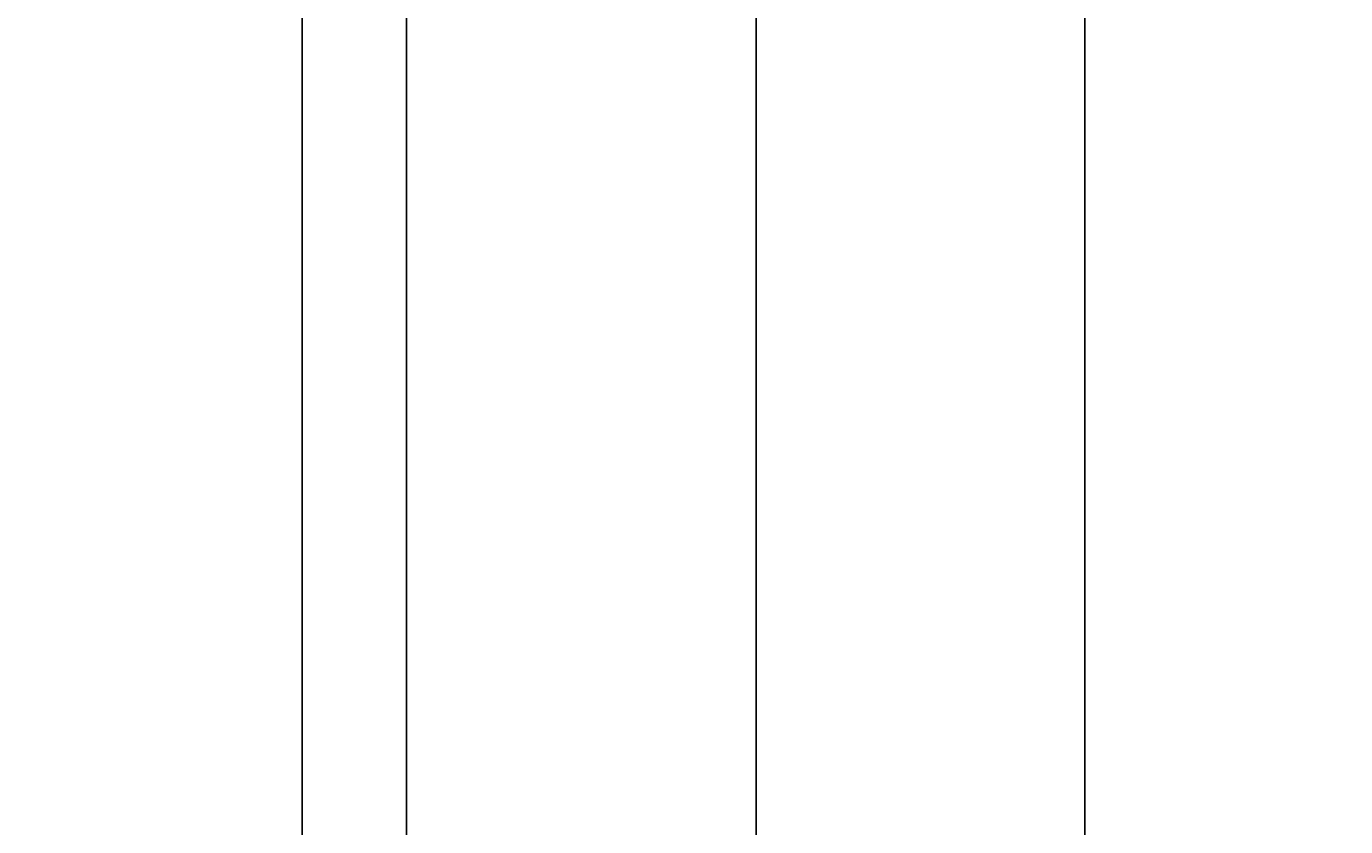
# Model space of a CAD drawing. Units: inches. Extents: x 2231 to 2461, y 2045 to 2455.
# Tile 54 of 95: x 2320 to 2371, y 2271 to 2302. Entities that reach past the tile are written whole.
import ezdxf

# ---------------------------------------------------------------- set-up
doc = ezdxf.new("R2010")
doc.units = ezdxf.units.IN
doc.layers.add('A-ANNO-DIMS', color=2, linetype='Continuous', lineweight=18)
doc.styles.get("Standard").update_dxf_attribs({"font": 'arial.ttf'})
doc.dimstyles.get("Standard").update_dxf_attribs({"dimtxt": 0.18, "dimasz": 0.18, "dimexe": 0.18, "dimexo": 0.0625, "dimgap": 0.09, "dimtad": 0, "dimtih": 1, "dimtoh": 1, "dimdec": 4, "dimzin": 0, "dimdsep": 46, "dimtxsty": 'Standard', "dimcen": 0.09, "dimadec": 0, "dimazin": 0, "dimtfac": 1, "dimtdec": 4, "dimtofl": 0, "dimtmove": 0, "dimatfit": 3, "dimfxl": 1, "dimtolj": 1, "dimtzin": 0, "dimarcsym": 0})

# ---------------------------------------------------------------- blocks, each defined once
blk = doc.blocks.new('*D50')
at = {"layer": 'A-ANNO-DIMS', "color": 0, "lineweight": -2, "transparency": 16777216}
for p, q in [((2304.794, 2182.895), (2304.794, 2454.645)), ((2334.794, 2182.895), (2334.794, 2454.645)), ((2304.974, 2454.465), (2319.575, 2454.465)), ((2334.614, 2454.465), (2320.012, 2454.465))]:
    blk.add_line(p, q, dxfattribs=at)
at = {"layer": 'A-ANNO-DIMS', "color": 0, "transparency": 16777216}
for points in [[(2304.974, 2454.495), (2304.974, 2454.435), (2304.794, 2454.465)], [(2334.614, 2454.495), (2334.614, 2454.435), (2334.794, 2454.465)]]:
    blk.add_solid(points, dxfattribs=at)
at = {"layer": 'Defpoints', "color": 0, "transparency": 16777216}
for p in [(2334.794, 2454.465), (2304.794, 2182.833), (2334.794, 2182.833)]:
    blk.add_point(p, dxfattribs=at)
at = {"layer": 'A-ANNO-DIMS', "color": 0, "transparency": 16777216, "insert": (2319.794, 2454.465), "char_height": 0.18, "attachment_point": 5}
blk.add_mtext('\\A1;30', dxfattribs=at)
blk = doc.blocks.new('*D51')
at = {"layer": 'A-ANNO-DIMS', "color": 0, "lineweight": -2, "transparency": 16777216}
for p, q in [((2258.794, 2306.77), (2258.794, 2044.803)), ((2330.794, 2306.77), (2330.794, 2044.803)), ((2258.974, 2044.983), (2294.576, 2044.983)), ((2330.614, 2044.983), (2295.011, 2044.983))]:
    blk.add_line(p, q, dxfattribs=at)
at = {"layer": 'A-ANNO-DIMS', "color": 0, "transparency": 16777216}
for points in [[(2258.974, 2045.013), (2258.974, 2044.953), (2258.794, 2044.983)], [(2330.614, 2045.013), (2330.614, 2044.953), (2330.794, 2044.983)]]:
    blk.add_solid(points, dxfattribs=at)
at = {"layer": 'Defpoints', "color": 0, "transparency": 16777216}
for p in [(2258.794, 2306.833), (2330.794, 2306.833), (2330.794, 2044.983)]:
    blk.add_point(p, dxfattribs=at)
at = {"layer": 'A-ANNO-DIMS', "color": 0, "transparency": 16777216, "insert": (2294.794, 2044.983), "char_height": 0.18, "attachment_point": 5}
blk.add_mtext('\\A1;72', dxfattribs=at)
blk = doc.blocks.new('*D52')
at = {"layer": 'A-ANNO-DIMS', "color": 0, "lineweight": -2, "transparency": 16777216}
for p, q in [((2330.794, 2306.77), (2330.794, 2044.803)), ((2360.794, 2306.77), (2360.794, 2044.803)), ((2330.974, 2044.983), (2345.575, 2044.983)), ((2360.614, 2044.983), (2346.012, 2044.983))]:
    blk.add_line(p, q, dxfattribs=at)
at = {"layer": 'A-ANNO-DIMS', "color": 0, "transparency": 16777216}
for points in [[(2330.974, 2045.013), (2330.974, 2044.953), (2330.794, 2044.983)], [(2360.614, 2045.013), (2360.614, 2044.953), (2360.794, 2044.983)]]:
    blk.add_solid(points, dxfattribs=at)
at = {"layer": 'Defpoints', "color": 0, "transparency": 16777216}
for p in [(2330.794, 2306.833), (2360.794, 2306.833), (2360.794, 2044.983)]:
    blk.add_point(p, dxfattribs=at)
at = {"layer": 'A-ANNO-DIMS', "color": 0, "transparency": 16777216, "insert": (2345.794, 2044.983), "char_height": 0.18, "attachment_point": 5}
blk.add_mtext('\\A1;30', dxfattribs=at)
blk = doc.blocks.new('*D66')
at = {"layer": 'A-ANNO-DIMS', "color": 0, "lineweight": -2, "transparency": 16777216}
for p, q in [((2348.189, 2096.895), (2348.189, 2454.645)), ((2408.794, 2096.895), (2408.794, 2454.645)), ((2348.369, 2454.465), (2378.167, 2454.465)), ((2408.614, 2454.465), (2378.815, 2454.465))]:
    blk.add_line(p, q, dxfattribs=at)
at = {"layer": 'A-ANNO-DIMS', "color": 0, "transparency": 16777216}
for points in [[(2348.369, 2454.495), (2348.369, 2454.435), (2348.189, 2454.465)], [(2408.614, 2454.495), (2408.614, 2454.435), (2408.794, 2454.465)]]:
    blk.add_solid(points, dxfattribs=at)
at = {"layer": 'Defpoints', "color": 0, "transparency": 16777216}
for p in [(2408.794, 2454.465), (2348.189, 2096.833), (2408.794, 2096.833)]:
    blk.add_point(p, dxfattribs=at)
at = {"layer": 'A-ANNO-DIMS', "color": 0, "transparency": 16777216, "insert": (2378.491, 2454.465), "char_height": 0.18, "attachment_point": 5}
blk.add_mtext('\\A1;60.6', dxfattribs=at)

msp = doc.modelspace()

# ---------------------------------------------------------------- dimensions: what is measured, and where the dimension line sits
at = {"layer": 'A-ANNO-DIMS'}
for base, p1, p2, override, picture, middle in [((2334.7935, 2454.4653), (2304.7935, 2182.8328), (2334.7935, 2182.8328), {"dimdec": 0, "dimlfac": 1, "dimrnd": 0, "dimzin": 0, "dimdsep": 46, "dimlunit": 2}, '*D50', (2319.7935, 2454.4653)), ((2408.7935, 2454.4653), (2348.1888, 2096.8328), (2408.7935, 2096.8328), {"dimdec": 1, "dimlfac": 1, "dimrnd": 0, "dimzin": 0, "dimdsep": 46, "dimlunit": 2}, '*D66', (2378.4912, 2454.4653)), ((2330.7935, 2044.9825), (2258.7935, 2306.8328), (2330.7935, 2306.8328), {"dimdec": 0, "dimlfac": 1, "dimrnd": 0, "dimzin": 0, "dimdsep": 46, "dimlunit": 2}, '*D51', (2294.7935, 2044.9825)), ((2360.7935, 2044.9825), (2330.7935, 2306.8328), (2360.7935, 2306.8328), {"dimdec": 0, "dimlfac": 1, "dimrnd": 0, "dimzin": 0, "dimdsep": 46, "dimlunit": 2}, '*D52', (2345.7935, 2044.9825))]:
    dim = msp.add_linear_dim(base=base, p1=p1, p2=p2, dimstyle='Standard', override=override, dxfattribs=at)
    dim.commit()
    dim.dimension.update_dxf_attribs({"geometry": picture, "text_midpoint": middle})

doc.saveas('drawing.dxf')
